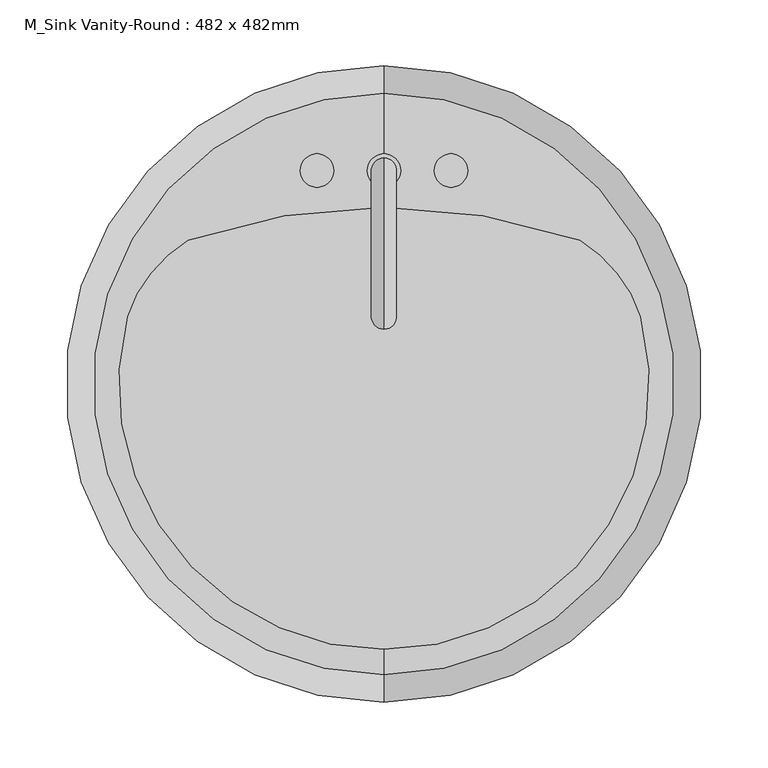
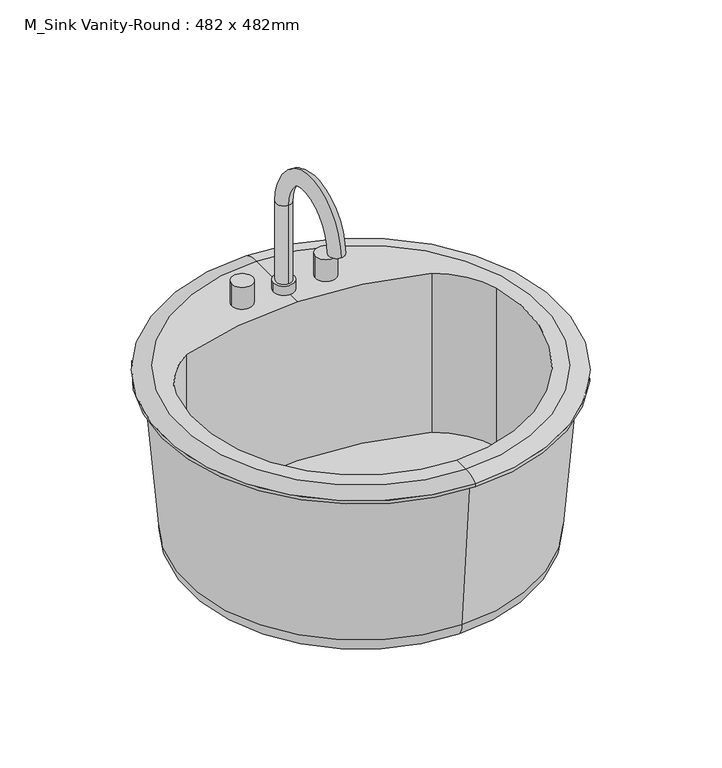
"""IFC4 building model written with IfcOpenShell, lengths in millimetres: flow terminal geometry, M_Sink Vanity-Round : 482 x 482mm."""

from ifc_helpers import new_model, si_unit, point, frame, frame_2d, origin, place, context, project, spatial, polyline, circle_curve, ellipse_curve, trimmed, segment, composite_curve, outline, extrude, source, transform, mapped, element, save
from ifc_brep_helpers import plane_surface, cylinder_surface, revolved_surface, advanced_brep


def m_sink_vanity_round_482_x_482mm_721ec264(model_context):
    return source(origin(), model_context, "Body", "SolidModel", [
        advanced_brep(
        [(96.6517406, -135.3870093, 759.525), (96.6517406, 305.7224463, 759.525), (96.6517406, 326.4677185, 753.96875), (96.6517406, -156.1322815, 753.96875), (96.6517406, -116.2405705, 759.525), (-98.1703414, 136.2525038, 759.525), (-52.1534933, 194.0861398, 759.525), (96.6517406, 219.2662048, 759.525), (245.4569744, 194.0861398, 759.525), (291.4738225, 136.2525038, 759.525), (96.6517406, -107.1264028, 534.1), (96.6517406, 277.4618398, 534.1), (96.6517406, 85.1677185, 534.1), (96.6517406, -127.6827361, 555.2842611), (96.6517406, 298.0181731, 555.2842611), (96.6517406, -144.2260315, 750.0), (96.6517406, 314.5614685, 750.0), (96.6517406, -156.1322815, 750.0), (96.6517406, 326.4677185, 750.0), (245.4569744, 194.0861398, 555.2842611), (-52.1534933, 194.0861398, 555.2842611), (-98.1703414, 136.2525038, 555.2842611), (291.4738225, 136.2525038, 555.2842611)],
        [
            (0, 1, circle_curve(frame((96.6517406, 85.1677185, 759.525), z_axis=(0.0, 0.0, -1.0), x_axis=(0.0, 1.0, 0.0)), 220.5547278)),
            (1, 2, circle_curve(frame((96.6517406, 309.4374616, 731.889434), z_axis=(-1.0, 0.0, 0.0), x_axis=(0.0, 1.0, 0.0)), 27.8841505)),
            (2, 3, circle_curve(frame((96.6517406, 85.1677185, 753.96875), z_axis=(0.0, 0.0, 1.0), x_axis=(0.0, 1.0, 0.0)), 241.3)),
            (3, 0, circle_curve(frame((96.6517406, -139.1020246, 731.889434), z_axis=(-1.0, 0.0, 0.0), x_axis=(0.0, -1.0, 0.0)), 27.8841505)),
            (1, 0, circle_curve(frame((96.6517406, 85.1677185, 759.525), z_axis=(0.0, 0.0, -1.0), x_axis=(0.0, 1.0, 0.0)), 220.5547278)),
            (3, 2, circle_curve(frame((96.6517406, 85.1677185, 753.96875), z_axis=(0.0, 0.0, 1.0), x_axis=(0.0, 1.0, 0.0)), 241.3)),
            (0, 4),
            (4, 5, circle_curve(frame((96.6517406, 85.1677185, 759.525), z_axis=(0.0, 0.0, -1.0), x_axis=(1.0, 0.0, 0.0)), 201.408289)),
            (5, 6, circle_curve(frame((1.3689689, 104.2755165, 759.525), z_axis=(0.0, 0.0, -1.0), x_axis=(1.0, 0.0, 0.0)), 104.5495194)),
            (6, 7, circle_curve(frame((96.6517406, -233.0168462, 759.525), z_axis=(0.0, 0.0, -1.0), x_axis=(1.0, 0.0, 0.0)), 452.283051)),
            (7, 1),
            (7, 8, circle_curve(frame((96.6517406, -233.0168462, 759.525), z_axis=(0.0, 0.0, -1.0), x_axis=(1.0, 0.0, 0.0)), 452.283051)),
            (8, 9, circle_curve(frame((191.9345122, 104.2755165, 759.525), z_axis=(0.0, 0.0, -1.0), x_axis=(1.0, 0.0, 0.0)), 104.5495194)),
            (9, 4, circle_curve(frame((96.6517406, 85.1677185, 759.525), z_axis=(0.0, 0.0, -1.0), x_axis=(1.0, 0.0, 0.0)), 201.408289)),
            (10, 11, circle_curve(frame((96.6517406, 85.1677185, 534.1), z_axis=(0.0, 0.0, -1.0), x_axis=(0.0, 1.0, 0.0)), 192.2941213)),
            (11, 12),
            (12, 10),
            (11, 10, circle_curve(frame((96.6517406, 85.1677185, 534.1), z_axis=(0.0, 0.0, -1.0), x_axis=(0.0, 1.0, 0.0)), 192.2941213)),
            (10, 13, circle_curve(frame((96.6517406, -107.1264028, 554.6656396), z_axis=(-1.0, 0.0, 0.0), x_axis=(0.0, -1.0, 0.0)), 20.5656396)),
            (13, 14, circle_curve(frame((96.6517406, 85.1677185, 555.2842611), z_axis=(0.0, 0.0, -1.0), x_axis=(0.0, 1.0, 0.0)), 212.8504546)),
            (14, 11, circle_curve(frame((96.6517406, 277.4618398, 554.6656396), z_axis=(-1.0, 0.0, 0.0), x_axis=(0.0, 1.0, 0.0)), 20.5656396)),
            (14, 13, circle_curve(frame((96.6517406, 85.1677185, 555.2842611), z_axis=(0.0, 0.0, -1.0), x_axis=(0.0, 1.0, 0.0)), 212.8504546)),
            (13, 15),
            (15, 16, circle_curve(frame((96.6517406, 85.1677185, 750.0), z_axis=(0.0, 0.0, -1.0), x_axis=(0.0, 1.0, 0.0)), 229.39375)),
            (16, 14),
            (16, 15, circle_curve(frame((96.6517406, 85.1677185, 750.0), z_axis=(0.0, 0.0, -1.0), x_axis=(0.0, 1.0, 0.0)), 229.39375)),
            (15, 17),
            (17, 18, circle_curve(frame((96.6517406, 85.1677185, 750.0), z_axis=(0.0, 0.0, -1.0), x_axis=(0.0, 1.0, 0.0)), 241.3)),
            (18, 16),
            (18, 17, circle_curve(frame((96.6517406, 85.1677185, 750.0), z_axis=(0.0, 0.0, -1.0), x_axis=(0.0, 1.0, 0.0)), 241.3)),
            (2, 18),
            (17, 3),
            (19, 20, circle_curve(frame((96.6517406, -233.0168462, 555.2842611), z_axis=(0.0, 0.0, 1.0), x_axis=(1.0, 0.0, 0.0)), 452.283051)),
            (20, 21, circle_curve(frame((1.3689689, 104.2755165, 555.2842611), z_axis=(0.0, 0.0, 1.0), x_axis=(1.0, 0.0, 0.0)), 104.5495194)),
            (21, 22, circle_curve(frame((96.6517406, 85.1677185, 555.2842611), z_axis=(0.0, 0.0, 1.0), x_axis=(1.0, 0.0, 0.0)), 201.408289)),
            (22, 19, circle_curve(frame((191.9345122, 104.2755165, 555.2842611), z_axis=(0.0, 0.0, 1.0), x_axis=(1.0, 0.0, 0.0)), 104.5495194)),
            (19, 8),
            (6, 20),
            (5, 21),
            (9, 22),
        ],
        [
            revolved_surface(trimmed(ellipse_curve(frame((96.6517406, 309.4374616, 731.889434), z_axis=(1.0, 0.0, 0.0), x_axis=(0.0, 1.0, 0.0)), 27.8841505, 27.8841505), [point((96.6517406, 326.4677185, 753.96875))], [point((96.6517406, 305.7224463, 759.525))], True, "CARTESIAN"), (96.6517406, 85.1677185, 759.525), (0.0, 0.0, 1.0)),
            plane_surface(frame((96.6517406, 85.1677185, 759.525), z_axis=(0.0, 0.0, 1.0), x_axis=(0.0, 1.0, 0.0))),
            plane_surface(frame((96.6517406, 85.1677185, 534.1), z_axis=(0.0, 0.0, -1.0), x_axis=(0.0, 1.0, 0.0))),
            revolved_surface(trimmed(ellipse_curve(frame((96.6517406, 277.4618398, 554.6656396), z_axis=(1.0, 0.0, 0.0), x_axis=(0.0, 1.0, 0.0)), 20.5656396, 20.5656396), [point((96.6517406, 277.4618398, 534.1))], [point((96.6517406, 298.0181731, 555.2842611))], True, "CARTESIAN"), (96.6517406, 85.1677185, 759.525), (0.0, 0.0, 1.0)),
            revolved_surface(polyline([(96.6517406, 298.0181731, 555.2842611), (96.6517406, 314.5614685, 750.0)]), (96.6517406, 85.1677185, 759.525), (0.0, 0.0, 1.0)),
            plane_surface(frame((96.6517406, 85.1677185, 750.0), z_axis=(0.0, 0.0, -1.0), x_axis=(0.0, 1.0, 0.0))),
            cylinder_surface(frame((96.6517406, 85.1677185, 759.525), z_axis=(0.0, 0.0, 1.0), x_axis=(0.0, 1.0, 0.0)), 241.3),
            plane_surface(frame((548.9347916, -233.0168462, 555.2842611), z_axis=(0.0, 0.0, 1.0), x_axis=(0.0, -1.0, 0.0))),
            revolved_surface(polyline([(548.9347916, -233.0168462, 759.525), (548.9347916, -233.0168462, 555.2842611)]), (96.6517406, -233.0168462, 555.2842611), (0.0, 0.0, 1.0)),
            revolved_surface(polyline([(105.91848829999999, 104.2755165, 759.525), (105.91848829999999, 104.2755165, 555.2842611)]), (1.3689689, 104.2755165, 555.2842611), (0.0, 0.0, 1.0)),
            revolved_surface(polyline([(298.0600296, 85.1677185, 759.525), (298.0600296, 85.1677185, 555.2842611)]), (96.6517406, 85.1677185, 555.2842611), (0.0, 0.0, 1.0)),
            revolved_surface(polyline([(296.4840316, 104.2755165, 759.525), (296.4840316, 104.2755165, 555.2842611)]), (191.9345122, 104.2755165, 555.2842611), (0.0, 0.0, 1.0)),
        ],
        [
            (0, [[1, 2, 3, 4]]),
            (0, [[-2, 5, -4, 6]]),
            (1, [[-1, 7, 8, 9, 10, 11]]),
            (1, [[-5, -11, 12, 13, 14, -7]]),
            (2, [[15, 16, 17]]),
            (2, [[-16, 18, -17]]),
            (3, [[-15, 19, 20, 21]]),
            (3, [[-18, -21, 22, -19]]),
            (4, [[-20, 23, 24, 25]]),
            (4, [[-22, -25, 26, -23]]),
            (5, [[-24, 27, 28, 29]]),
            (5, [[-26, -29, 30, -27]]),
            (6, [[-3, 31, -28, 32]]),
            (6, [[-6, -32, -30, -31]]),
            (7, [[33, 34, 35, 36]]),
            (8, [[-33, 37, -12, -10, 38]]),
            (9, [[-34, -38, -9, 39]]),
            (10, [[-35, -39, -8, -14, 40]]),
            (11, [[-36, -40, -13, -37]]),
        ],
    ),
        extrude(outline(composite_curve([segment(trimmed(circle_curve(frame_2d((147.4517406, 247.0927185)), 12.7), [point((134.7517406, 247.0927185))], [point((160.1517406, 247.0927185))], False, "CARTESIAN"), True, "CONTINUOUS"), segment(trimmed(circle_curve(frame_2d((147.4517406, 247.0927185)), 12.7), [point((160.1517406, 247.0927185))], [point((134.7517406, 247.0927185))], False, "CARTESIAN"), True, "CONTINUOUS")], self_intersect=False)), frame((0.0, 0.0, 759.525), z_axis=(0.0, 0.0, 1.0), x_axis=(1.0, 0.0, 0.0)), (0.0, 0.0, 1.0), 28.575),
        extrude(outline(composite_curve([segment(trimmed(circle_curve(frame_2d((45.8517406, 247.0927185)), 12.7), [point((33.1517406, 247.0927185))], [point((58.5517406, 247.0927185))], False, "CARTESIAN"), True, "CONTINUOUS"), segment(trimmed(circle_curve(frame_2d((45.8517406, 247.0927185)), 12.7), [point((58.5517406, 247.0927185))], [point((33.1517406, 247.0927185))], False, "CARTESIAN"), True, "CONTINUOUS")], self_intersect=False)), frame((0.0, 0.0, 759.525), z_axis=(0.0, 0.0, 1.0), x_axis=(1.0, 0.0, 0.0)), (0.0, 0.0, 1.0), 28.575),
        advanced_brep(
        [(83.9517406, 247.0927185, 771.7602909), (109.3517406, 247.0927185, 771.7602909), (96.6517406, 237.5677185, 771.7602909), (96.6517406, 256.6177185, 771.7602909), (83.9517406, 247.0927185, 759.525), (109.3517406, 247.0927185, 759.525), (96.6517406, 237.5677185, 872.2375), (96.6517406, 256.6177185, 872.2375), (96.6517406, 145.7775038, 872.2375), (96.6517406, 126.7275038, 872.2375)],
        [
            (0, 1, circle_curve(frame((96.6517406, 247.0927185, 771.7602909), z_axis=(0.0, 0.0, 1.0), x_axis=(1.0, 0.0, 0.0)), 12.7)),
            (1, 0, circle_curve(frame((96.6517406, 247.0927185, 771.7602909), z_axis=(0.0, 0.0, 1.0), x_axis=(1.0, 0.0, 0.0)), 12.7)),
            (2, 3, circle_curve(frame((96.6517406, 247.0927185, 771.7602909), z_axis=(0.0, 0.0, -1.0), x_axis=(0.0, 1.0, 0.0)), 9.525)),
            (3, 2, circle_curve(frame((96.6517406, 247.0927185, 771.7602909), z_axis=(0.0, 0.0, -1.0), x_axis=(0.0, 1.0, 0.0)), 9.525)),
            (4, 5, circle_curve(frame((96.6517406, 247.0927185, 759.525), z_axis=(0.0, 0.0, -1.0), x_axis=(1.0, 0.0, 0.0)), 12.7)),
            (5, 4, circle_curve(frame((96.6517406, 247.0927185, 759.525), z_axis=(0.0, 0.0, -1.0), x_axis=(1.0, 0.0, 0.0)), 12.7)),
            (0, 4),
            (5, 1),
            (6, 7, circle_curve(frame((96.6517406, 247.0927185, 872.2375), z_axis=(0.0, 0.0, -1.0), x_axis=(0.0, 1.0, 0.0)), 9.525)),
            (7, 3),
            (2, 6),
            (7, 6, circle_curve(frame((96.6517406, 247.0927185, 872.2375), z_axis=(0.0, 0.0, -1.0), x_axis=(0.0, 1.0, 0.0)), 9.525)),
            (8, 9, circle_curve(frame((96.6517406, 136.2525038, 872.2375), z_axis=(0.0, 0.0, -1.0), x_axis=(0.0, -1.0, 0.0)), 9.525)),
            (9, 8, circle_curve(frame((96.6517406, 136.2525038, 872.2375), z_axis=(0.0, 0.0, -1.0), x_axis=(0.0, -1.0, 0.0)), 9.525)),
            (6, 8, circle_curve(frame((96.6517406, 191.6726112, 872.2375), z_axis=(1.0, 0.0, 0.0), x_axis=(0.0, 1.0, 0.0)), 45.8951073)),
            (9, 7, circle_curve(frame((96.6517406, 191.6726112, 872.2375), z_axis=(-1.0, 0.0, 0.0), x_axis=(0.0, 1.0, 0.0)), 64.9451073)),
        ],
        [
            plane_surface(frame((109.3517406, 247.0927185, 771.7602909), z_axis=(0.0, 0.0, 1.0), x_axis=(0.0, 1.0, 0.0))),
            plane_surface(frame((109.3517406, 247.0927185, 759.525), z_axis=(0.0, 0.0, -1.0), x_axis=(0.0, -1.0, 0.0))),
            cylinder_surface(frame((96.6517406, 247.0927185, 759.525), z_axis=(0.0, 0.0, 1.0), x_axis=(1.0, 0.0, 0.0)), 12.7),
            cylinder_surface(frame((96.6517406, 247.0927185, 759.525), z_axis=(0.0, 0.0, -1.0), x_axis=(0.0, 1.0, 0.0)), 9.525),
            plane_surface(frame((96.6517406, 191.6726112, 872.2375), z_axis=(0.0, 0.0, -1.0), x_axis=(0.0, -1.0, 0.0))),
            revolved_surface(trimmed(ellipse_curve(frame((96.6517406, 247.0927185, 872.2375), z_axis=(0.0, 0.0, -1.0), x_axis=(0.0, 1.0, 0.0)), 9.525, 9.525), [point((96.6517406, 237.5677185, 872.2375))], [point((96.6517406, 256.6177185, 872.2375))], True, "CARTESIAN"), (96.6517406, 191.6726112, 872.2375), (1.0, 0.0, 0.0)),
            revolved_surface(trimmed(ellipse_curve(frame((96.6517406, 247.0927185, 872.2375), z_axis=(0.0, 0.0, -1.0), x_axis=(0.0, 1.0, 0.0)), 9.525, 9.525), [point((96.6517406, 256.6177185, 872.2375))], [point((96.6517406, 237.5677185, 872.2375))], True, "CARTESIAN"), (96.6517406, 191.6726112, 872.2375), (1.0, 0.0, 0.0)),
        ],
        [
            (0, [[1, 2], [3, 4]]),
            (1, [[5, 6]]),
            (2, [[-1, 7, -6, 8]]),
            (2, [[-2, -8, -5, -7]]),
            (3, [[9, 10, -3, 11]]),
            (3, [[12, -11, -4, -10]]),
            (4, [[13, 14]]),
            (5, [[-9, 15, -14, 16]]),
            (6, [[-12, -16, -13, -15]]),
        ],
    ),
    ])


if __name__ == "__main__":
    model = new_model("IFC4")
    model_context = context("Model", 3, world=origin())
    ifc_project = project(units=[si_unit("LENGTHUNIT", "METRE", prefix="MILLI")], contexts=[model_context])
    site = spatial("IfcSite", under=ifc_project)
    building = spatial("IfcBuilding", under=site)
    placement = place(None, origin())
    m_sink_vanity_round_482_x_482mm_shape = m_sink_vanity_round_482_x_482mm_721ec264(model_context)
    element("IfcFlowTerminal", 1, ObjectType="M_Sink Vanity-Round : 482 x 482mm", at=placement, inside=building, context=model_context, shape_type="MappedRepresentation", body=[
        mapped(m_sink_vanity_round_482_x_482mm_shape, transform((0.0, 0.0, 0.0), x_axis=(1.0, 0.0, 0.0), y_axis=(0.0, 1.0, 0.0), z_axis=(0.0, 0.0, 1.0))),
    ])
    save(model, "model.ifc")

# Revit data of these elements
# Type "M_Sink Vanity-Round : 482 x 482mm"
#   Top Of Counter [instance default] = 750 mm
#   Basin Material = Porcelain, Linen
#   Fixture Material = Steel, Polished
#   Default Elevation = 0
# Element 1 (IfcFlowTerminal, "M_Sink Vanity-Round : 482 x 482mm")
#   Materials on its faces: "Porcelain, Linen", "Steel, Polished"
# Materials
#   "Porcelain, Linen": class "Ceramic", colour RGB 249 239 230, transparency 0, Description = "Porcelain, linen", Cost = 0
#   "Steel, Polished": class "Metal", colour RGB 57 57 57, transparency 0, Description = "Polished steel", Cost = 0
